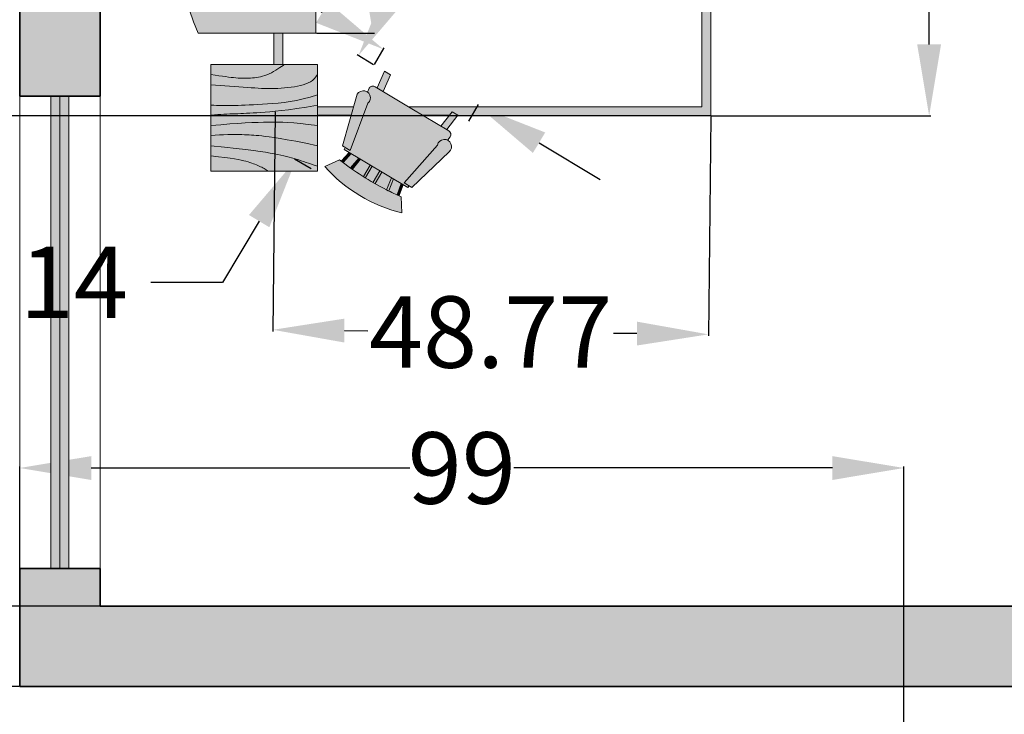
# Model space of a CAD drawing. Units: inches. Extents: x -52 to 678, y 23 to 685.
# Tile 3 of 11: x 189 to 299, y 143 to 221. Entities that reach past the tile are written whole.
import ezdxf

# ---------------------------------------------------------------- set-up
doc = ezdxf.new("R2010")
doc.units = ezdxf.units.IN
doc.header["$MEASUREMENT"] = 0
for name, color, linetype, lineweight in [('A-ANNO-DIMS', 2, 'Continuous', 18), ('A-FLOR', 7, 'Continuous', 25), ('A-FURN', 8, 'Continuous', 18), ('A-FURN-PATT', 252, 'Continuous', 13), ('A-GLAZ', 4, 'Continuous', 18), ('A-WALL', 7, 'Continuous', 35)]:
    doc.layers.add(name, color=color, linetype=linetype, lineweight=lineweight)
doc.layers.add('A-GLAZ-PATT', color=18, linetype='Continuous', lineweight=13, true_color=0x000000)
doc.layers.add('A-WALL-PATT', color=18, linetype='Continuous', lineweight=13, true_color=0x000000)
doc.styles.get("Standard").update_dxf_attribs({"font": 'arial.ttf'})
doc.dimstyles.get("Standard").update_dxf_attribs({"dimtxt": 8, "dimasz": 8, "dimexe": 0.18, "dimexo": 0.0625, "dimgap": 0.09, "dimtad": 0, "dimtih": 1, "dimtoh": 1, "dimdec": 0, "dimzin": 0, "dimdsep": 46, "dimlunit": 3, "dimtxsty": 'Standard', "dimcen": 0.09, "dimadec": 0, "dimazin": 0, "dimtfac": 1, "dimtdec": 0, "dimtofl": 0, "dimtmove": 0, "dimatfit": 3, "dimfxl": 1, "dimtolj": 1, "dimtzin": 0, "dimarcsym": 0})

# ---------------------------------------------------------------- blocks, each defined once
blk = doc.blocks.new('Table - Square Woodgrain 42 x 42 in.')
blk.add_line((0, -42), (42, -42))
for points in [[(0, -4), (1.704, -4.2172), (3.2358, -4.4188), (4.615, -4.604), (5.8615, -4.7721), (6.9951, -4.9224), (8.0357, -5.0541), (9.0031, -5.1667), (9.9171, -5.2594), (10.7951, -5.3316), (11.6445, -5.3836), (12.4702, -5.4157), (13.277, -5.4283), (14.0698, -5.4217), (14.8535, -5.3964), (15.6331, -5.3526), (16.4133, -5.2908), (17.1986, -5.2103), (17.9913, -5.1062), (18.793, -4.9727), (19.6056, -4.8038), (20.4307, -4.5937), (21.2701, -4.3365), (22.1256, -4.0262), (22.9989, -3.6571), (23.888, -3.2272), (24.7756, -2.7516), (25.6408, -2.2491), (26.4624, -1.7387), (27.2195, -1.2395), (27.891, -0.7703), (28.456, -0.3501), (28.8934, 0.002)], [(0, -42), (0, 0), (42, 0), (42, -42)], [(0, -8), (1.8203, -8.1001), (3.6741, -8.2149), (5.5411, -8.3408), (7.4011, -8.4741), (9.2339, -8.6112), (11.0193, -8.7484), (12.7371, -8.8821), (14.3671, -9.0086), (15.8954, -9.1246), (17.3337, -9.2278), (18.6997, -9.3159), (20.0116, -9.387), (21.2871, -9.4389), (22.5442, -9.4696), (23.8008, -9.477), (25.0749, -9.459), (26.3791, -9.4137), (27.7049, -9.3403), (29.0383, -9.2382), (30.3655, -9.1068), (31.6728, -8.9455), (32.9461, -8.7535), (34.1717, -8.5304), (35.3358, -8.2756), (36.4268, -7.9863), (37.443, -7.6521), (38.3849, -7.2603), (39.253, -6.7986), (40.048, -6.2542), (40.7705, -5.6147), (41.421, -4.8674), (42, -4)], [(42, -12), (39.1784, -12.8621), (36.4519, -13.5654), (33.8246, -14.1294), (31.3004, -14.5731), (28.8832, -14.9161), (26.577, -15.1775), (24.3858, -15.3768), (22.3136, -15.5332), (20.3622, -15.6632), (18.5254, -15.7718), (16.7947, -15.8612), (15.1618, -15.9338), (13.6183, -15.9916), (12.1558, -16.0369), (10.7659, -16.0718), (9.4403, -16.0987), (8.1703, -16.1191), (6.9461, -16.1325), (5.7577, -16.1377), (4.595, -16.1335), (3.4479, -16.1188), (2.3064, -16.0924), (1.1604, -16.0532), (0, -16)], [(42, -16), (37.6529, -16.7365), (33.8802, -17.329), (30.6179, -17.7961), (27.8015, -18.1561), (25.3668, -18.4275), (23.2497, -18.6288), (21.3859, -18.7785), (19.7111, -18.8949), (18.1693, -18.9939), (16.7375, -19.0795), (15.401, -19.1534), (14.1449, -19.217), (12.9544, -19.2717), (11.8148, -19.3191), (10.7113, -19.3606), (9.6291, -19.3976), (8.5534, -19.4323), (7.47, -19.4689), (6.3643, -19.5122), (5.222, -19.5672), (4.0288, -19.6386), (2.7703, -19.7313), (1.4321, -19.8501), (0, -20)], [(0, -24), (3.9243, -23.6805), (7.4766, -23.4138), (10.6891, -23.1954), (13.5943, -23.0205), (16.2247, -22.8847), (18.6125, -22.7832), (20.7903, -22.7116), (22.7903, -22.6651), (24.6563, -22.642), (26.4764, -22.6507), (28.35, -22.7024), (30.3766, -22.8084), (32.6555, -22.98), (35.2861, -23.2283), (38.3678, -23.5645), (42, -24)], [(42, -32), (37.392, -31.017), (33.4585, -30.2231), (30.1291, -29.5949), (27.3334, -29.109), (25.0009, -28.742), (23.0612, -28.4707), (21.4439, -28.2716), (20.0786, -28.1215), (18.8998, -28.0002), (17.8609, -27.9014), (16.9206, -27.8219), (16.0371, -27.7588), (15.1691, -27.709), (14.2748, -27.6693), (13.3128, -27.6368), (12.2415, -27.6083), (11.0295, -27.5824), (9.6867, -27.5643), (8.233, -27.5608), (6.6884, -27.5787), (5.0728, -27.6248), (3.4062, -27.7058), (1.7086, -27.8286), (0, -28)], [(0, -32), (5.4026, -32.5358), (9.9494, -33.019), (13.7424, -33.4553), (16.8834, -33.8505), (19.4743, -34.2106), (21.6171, -34.5413), (23.4136, -34.8486), (24.9657, -35.1382), (26.3614, -35.4156), (27.6332, -35.6841), (28.7995, -35.9467), (29.8788, -36.2064), (30.8897, -36.4661), (31.8507, -36.7288), (32.7802, -36.9973), (33.6968, -37.2747), (34.6175, -37.5635), (35.5531, -37.8651), (36.5128, -38.1805), (37.506, -38.5108), (38.5421, -38.8568), (39.6302, -39.2197), (40.7797, -39.6004), (42, -40)], [(0, -36), (3.0098, -36.2857), (5.5354, -36.5643), (7.6368, -36.8359), (9.374, -37.1009), (10.807, -37.3597), (11.9957, -37.6126), (13.0002, -37.8599), (13.8804, -38.102), (14.6874, -38.3393), (15.4365, -38.5729), (16.1338, -38.8041), (16.7858, -39.0341), (17.3987, -39.264), (17.9787, -39.4952), (18.5322, -39.7288), (19.0655, -39.9662), (19.5832, -40.2081), (20.0842, -40.4544), (20.5657, -40.7046), (21.0249, -40.9581), (21.459, -41.2144), (21.8653, -41.4731), (22.2409, -41.7335), (22.5831, -41.9951)]]:
    blk.add_lwpolyline(points)
blk = doc.blocks.new('Chair - Rocking')
for p, q in [((-8, -4.5), (-10, -1.5)), ((8, -4.5), (10, -1.5)), ((-4.5, -7), (-4.96674, -4.19951)), ((-4, -7), (-4.40532, -4.16272)), ((-1.5, -4.05012), (-1.5, -7)), ((-1, -7), (-1, -4.05012)), ((1, -7), (1, -4.04655)), ((1.5, -4.05012), (1.5, -7)), ((4, -7), (4.40187, -4.18694)), ((4.5, -7), (4.96761, -4.19437)), ((-7.5, -4.5), (-7, -7)), ((-6.5, -7), (-7.02225, -4.43)), ((6.5, -7), (7, -4.4057)), ((7.5, -4.5), (7, -7)), ((-9, -7.5), (-12, -18.49999)), ((-7, -7.5), (-9, -7.5)), ((-9, -18.49999), (-7, -7.5)), ((-8.23428, -6.99939), (-8.3093, -7.47958)), ((-8.23041, -7), (8.23915, -7)), ((7, -7.5), (9, -7.5)), ((9, -18.49999), (7, -7.5)), ((8.31071, -7.48854), (8.23449, -7.00073)), ((9, -7.5), (12, -18.49999)), ((-10.36644, -20.64523), (-10.5, -21.49999)), ((10.5, -21.49999), (10.3575, -20.58798)), ((-9, -22.49999), (-9.5, -26.49999)), ((0, -22.49999), (-9.5, -22.49999)), ((-8, -26.49999), (-7.5, -22.49999)), ((0, -22.49999), (9.5, -22.49999)), ((8, -26.49999), (7.5, -22.49999)), ((9, -22.49999), (9.5, -26.49999)), ((-9.5, -26.49999), (-8, -26.49999)), ((9.5, -26.49999), (8, -26.49999))]:
    blk.add_line(p, q)
for centre, radius, start, end in [((0, -34.08333), 34.08333, 72.93847, 107.0615), ((0, -68.25004), 64.25, 93.92211, 97.15267), ((0, -68.25004), 64.25, 82.84733, 93.92211), ((-10.5, -18.99999), 1.58114, 161.5651, 18.43495), ((10.5, -18.99999), 1.58114, 161.5651, 18.43495), ((-9.5, -21.49999), 1, 180, 270), ((9.5, -21.49999), 1, 270, 0)]:
    blk.add_arc(centre, radius, start, end)
blk = doc.blocks.new('Sofa - Roundback 7 ft.')
for p, q in [((-12.00002, -32.4421), (-12.00003, -6.5971)), ((11.99997, -32.4421), (11.99998, -6.5971)), ((-36.000027, -34), (-36.000027, -11.4696)), ((35.99998, -34), (35.99998, -11.4696)), ((-35.999844, -13.3819), (35.9998, -13.3819)), ((-36.000027, -32.4421), (35.99998, -32.4421))]:
    blk.add_line(p, q)
for points in [[(-36.000027, -34), (-42.000027, -34), (-42.000027, -8)], [(41.99998, -8), (41.99998, -34), (35.99998, -34)]]:
    blk.add_lwpolyline(points)
for centre, radius, start, end in [((0, -114.25), 114.25, 68.43141, 111.5686), ((-0.00001, -127.1968), 121.1968, 72.72033, 107.2797)]:
    blk.add_arc(centre, radius, start, end)
blk = doc.blocks.new('*D21')
at = {"layer": 'A-ANNO-DIMS', "color": 0, "lineweight": -2, "transparency": 16777216}
for p, q in [((230.65, 223.62), (234.77, 230.48)), ((228.24, 215.74), (226.38, 216.85)), ((221.23, 204.07), (219.38, 205.18)), ((215.42, 198.23), (211.3, 191.37)), ((211.3, 191.37), (203.3, 191.37))]:
    blk.add_line(p, q, dxfattribs=at)
at = {"layer": 'A-ANNO-DIMS', "color": 0, "transparency": 16777216}
for points in [[(229.51, 224.3), (231.8, 222.93), (226.54, 216.76)], [(214.28, 198.91), (216.56, 197.54), (219.54, 205.09)]]:
    blk.add_solid(points, dxfattribs=at)
at = {"layer": 'Defpoints', "color": 0, "transparency": 16777216}
for p in [(228.29, 215.71), (219.54, 205.09), (221.29, 204.04)]:
    blk.add_point(p, dxfattribs=at)
at = {"layer": 'A-ANNO-DIMS', "color": 0, "transparency": 16777216, "insert": (172.25, 191.37), "char_height": 8, "attachment_point": 5}
blk.add_mtext('\\A1;ROCKER 14', dxfattribs=at)
blk = doc.blocks.new('*D22')
at = {"layer": 'A-ANNO-DIMS', "color": 0, "lineweight": -2, "transparency": 16777216}
for p, q in [((215.62, 225.69), (207.62, 225.69)), ((222.48, 221.57), (215.62, 225.69)), ((228.32, 215.76), (229.43, 217.61)), ((238.88, 209.42), (239.99, 211.27)), ((246.76, 207), (253.62, 202.89))]:
    blk.add_line(p, q, dxfattribs=at)
at = {"layer": 'A-ANNO-DIMS', "color": 0, "transparency": 16777216}
for points in [[(223.17, 222.72), (221.79, 220.43), (229.34, 217.46)], [(247.45, 208.15), (246.07, 205.86), (239.9, 211.12)]]:
    blk.add_solid(points, dxfattribs=at)
at = {"layer": 'Defpoints', "color": 0, "transparency": 16777216}
for p in [(229.34, 217.46), (228.29, 215.71), (238.85, 209.37)]:
    blk.add_point(p, dxfattribs=at)
at = {"layer": 'A-ANNO-DIMS', "color": 0, "transparency": 16777216, "insert": (202.22, 225.69), "char_height": 8, "attachment_point": 5}
blk.add_mtext('\\A1;12', dxfattribs=at)
blk = doc.blocks.new('*D25')
at = {"layer": 'A-ANNO-DIMS', "color": 0, "lineweight": -2, "transparency": 16777216}
for p, q in [((221.83, 261.88), (228.34, 261.88)), ((228.16, 253.88), (228.16, 244.8)), ((228.16, 227.25), (228.16, 236.33)), ((221.83, 219.25), (228.34, 219.25))]:
    blk.add_line(p, q, dxfattribs=at)
at = {"layer": 'A-ANNO-DIMS', "color": 0, "transparency": 16777216}
for points in [[(226.83, 253.88), (229.49, 253.88), (228.16, 261.88)], [(226.83, 227.25), (229.49, 227.25), (228.16, 219.25)]]:
    blk.add_solid(points, dxfattribs=at)
at = {"layer": 'Defpoints', "color": 0, "transparency": 16777216}
for p in [(221.77, 261.88), (228.16, 261.88), (221.77, 219.25)]:
    blk.add_point(p, dxfattribs=at)
at = {"layer": 'A-ANNO-DIMS', "color": 0, "transparency": 16777216, "insert": (228.16, 240.57), "char_height": 8, "attachment_point": 5}
blk.add_mtext('\\A1;SOFA 43', dxfattribs=at)
blk = doc.blocks.new('*D39')
at = {"layer": 'A-ANNO-DIMS', "color": 0, "lineweight": -2, "transparency": 16777216}
for p, q in [((91.61, 327.06), (91.61, 28.49)), ((575.61, 53.06), (575.61, 28.49)), ((99.61, 28.67), (324.53, 28.67)), ((567.61, 28.67), (342.68, 28.67))]:
    blk.add_line(p, q, dxfattribs=at)
at = {"layer": 'A-ANNO-DIMS', "color": 0, "transparency": 16777216}
for points in [[(99.61, 30), (99.61, 27.33), (91.61, 28.67)], [(567.61, 30), (567.61, 27.33), (575.61, 28.67)]]:
    blk.add_solid(points, dxfattribs=at)
at = {"layer": 'Defpoints', "color": 0, "transparency": 16777216}
for p in [(91.61, 327.13), (575.61, 53.13), (575.61, 28.67)]:
    blk.add_point(p, dxfattribs=at)
at = {"layer": 'A-ANNO-DIMS', "color": 0, "transparency": 16777216, "insert": (333.61, 28.67), "char_height": 8, "attachment_point": 5}
blk.add_mtext('\\A1;484', dxfattribs=at)
blk = doc.blocks.new('*D47')
at = {"layer": 'A-ANNO-DIMS', "color": 0, "lineweight": -2, "transparency": 16777216}
for p, q in [((188.54, 146.13), (66.97, 146.13)), ((67.15, 138.13), (67.15, 103.8)), ((67.15, 61.13), (67.15, 95.45)), ((425.54, 53.13), (66.97, 53.13))]:
    blk.add_line(p, q, dxfattribs=at)
at = {"layer": 'A-ANNO-DIMS', "color": 0, "transparency": 16777216}
for points in [[(65.81, 138.13), (68.48, 138.13), (67.15, 146.13)], [(65.81, 61.13), (68.48, 61.13), (67.15, 53.13)]]:
    blk.add_solid(points, dxfattribs=at)
at = {"layer": 'Defpoints', "color": 0, "transparency": 16777216}
for p in [(67.15, 146.13), (188.61, 146.13), (425.61, 53.13)]:
    blk.add_point(p, dxfattribs=at)
at = {"layer": 'A-ANNO-DIMS', "color": 0, "transparency": 16777216, "insert": (67.15, 99.63), "char_height": 8, "attachment_point": 5}
blk.add_mtext('\\A1;93', dxfattribs=at)
blk = doc.blocks.new('*D49')
at = {"layer": 'A-ANNO-DIMS', "color": 0, "lineweight": -2, "transparency": 16777216}
for p, q in [((188.61, 146.19), (188.61, 170.77)), ((196.61, 170.59), (232.28, 170.59)), ((279.61, 170.59), (243.93, 170.59)), ((287.61, 146.19), (287.61, 170.77))]:
    blk.add_line(p, q, dxfattribs=at)
at = {"layer": 'A-ANNO-DIMS', "color": 0, "transparency": 16777216}
for points in [[(196.61, 171.92), (196.61, 169.25), (188.61, 170.59)], [(279.61, 171.92), (279.61, 169.25), (287.61, 170.59)]]:
    blk.add_solid(points, dxfattribs=at)
at = {"layer": 'Defpoints', "color": 0, "transparency": 16777216}
for p in [(287.61, 170.59), (188.61, 146.13), (287.61, 146.13)]:
    blk.add_point(p, dxfattribs=at)
at = {"layer": 'A-ANNO-DIMS', "color": 0, "transparency": 16777216, "insert": (238.11, 170.59), "char_height": 8, "attachment_point": 5}
blk.add_mtext('\\A1;99', dxfattribs=at)
blk = doc.blocks.new('*D101')
at = {"layer": 'A-ANNO-DIMS', "color": 0, "lineweight": -2, "transparency": 16777216}
for p, q in [((217.21, 210.45), (216.96, 185.88)), ((265.98, 209.95), (265.72, 185.37)), ((224.96, 185.98), (227.59, 185.95)), ((257.72, 185.64), (255.09, 185.66))]:
    blk.add_line(p, q, dxfattribs=at)
at = {"layer": 'A-ANNO-DIMS', "color": 0, "transparency": 16777216}
for points in [[(224.97, 187.31), (224.94, 184.64), (216.96, 186.06)], [(257.74, 186.97), (257.71, 184.3), (265.72, 185.55)]]:
    blk.add_solid(points, dxfattribs=at)
at = {"layer": 'Defpoints', "color": 0, "transparency": 16777216}
for p in [(217.21, 210.52), (265.98, 210.01), (216.96, 186.06)]:
    blk.add_point(p, dxfattribs=at)
at = {"layer": 'A-ANNO-DIMS', "color": 0, "transparency": 16777216, "insert": (241.34, 185.81), "char_height": 8, "attachment_point": 5}
blk.add_mtext('\\A1;48.77', dxfattribs=at)
blk = doc.blocks.new('*D102')
at = {"layer": 'A-ANNO-DIMS', "color": 0, "lineweight": -2, "transparency": 16777216}
for p, q in [((266.04, 271.64), (290.62, 271.64)), ((290.44, 263.64), (290.44, 245)), ((290.44, 218.01), (290.44, 236.65)), ((266.04, 210.01), (290.62, 210.01))]:
    blk.add_line(p, q, dxfattribs=at)
at = {"layer": 'A-ANNO-DIMS', "color": 0, "transparency": 16777216}
for points in [[(289.1, 263.64), (291.77, 263.64), (290.44, 271.64)], [(289.1, 218.01), (291.77, 218.01), (290.44, 210.01)]]:
    blk.add_solid(points, dxfattribs=at)
at = {"layer": 'Defpoints', "color": 0, "transparency": 16777216}
for p in [(265.98, 271.64), (265.98, 210.01), (290.44, 210.01)]:
    blk.add_point(p, dxfattribs=at)
at = {"layer": 'A-ANNO-DIMS', "color": 0, "transparency": 16777216, "insert": (290.44, 240.82), "char_height": 8, "attachment_point": 5}
blk.add_mtext('\\A1;61.63', dxfattribs=at)
blk = doc.blocks.new('*D104')
at = {"layer": 'A-ANNO-DIMS', "color": 0, "lineweight": -2, "transparency": 16777216}
for p, q in [((265.91, 210.01), (66.97, 210.01)), ((67.15, 202.01), (67.15, 186.74)), ((67.15, 163.13), (67.15, 178.39)), ((301.21, 155.13), (66.97, 155.13))]:
    blk.add_line(p, q, dxfattribs=at)
at = {"layer": 'A-ANNO-DIMS', "color": 0, "transparency": 16777216}
for points in [[(65.81, 202.01), (68.48, 202.01), (67.15, 210.01)], [(65.81, 163.13), (68.48, 163.13), (67.15, 155.13)]]:
    blk.add_solid(points, dxfattribs=at)
at = {"layer": 'Defpoints', "color": 0, "transparency": 16777216}
for p in [(265.98, 210.01), (67.15, 155.13), (301.27, 155.13)]:
    blk.add_point(p, dxfattribs=at)
at = {"layer": 'A-ANNO-DIMS', "color": 0, "transparency": 16777216, "insert": (67.15, 182.57), "char_height": 8, "attachment_point": 5}
blk.add_mtext('\\A1;54.89', dxfattribs=at)

msp = doc.modelspace()

# ---------------------------------------------------------------- hatches: boundary and pattern name
at = {"layer": 'A-FURN-PATT'}
h = msp.add_hatch(color=256, dxfattribs=at)
h.dxf.hatch_style = 1
h.paths.add_polyline_path([(264.9763, 211.0118), (232.1935, 211.0118), (232.532, 210.8087), (233.7567, 210.0739), (236.7223, 210.0739), (237.0272, 210.4629), (237.6755, 210.0739), (265.9763, 210.0118), (265.9763, 211.0118), (265.9763, 271.638), (264.9763, 271.638), (252.0267, 271.638), (252.0267, 270.638), (264.9763, 270.638)])
h = msp.add_hatch(color=256, dxfattribs=at)
h.dxf.hatch_style = 1
h.paths.add_polyline_path([(221.7669, 219.2523), (221.7669, 222.2971), (210.3335, 222.2971, -0.15194781), (210.3335, 258.8353), (221.7669, 258.8353), (221.7669, 261.8802), (208.5725, 261.8802, 0.19047621), (208.5725, 219.2523)])
h = msp.add_hatch(color=256, dxfattribs=at)
h.dxf.hatch_style = 1
h.paths.add_polyline_path([(218.0681, 219.2523), (217.0681, 219.2523), (217.0681, 215.7592), (218.0681, 215.7592)])
h = msp.add_hatch(color=256, dxfattribs=at)
h.dxf.hatch_style = 1
h.paths.add_polyline_path([(214.8875, 214.2771), (215.113, 214.3067), (215.3411, 214.3447), (215.5722, 214.3927), (215.8069, 214.4525), (216.0457, 214.5257), (216.2891, 214.6139), (216.5375, 214.7189), (216.7904, 214.8412), (217.0429, 214.9765), (217.289, 215.1195), (217.5227, 215.2646), (217.7381, 215.4066), (217.9291, 215.5401), (218.0898, 215.6596), (218.2135, 215.7592), (209.9953, 215.7592), (209.9953, 214.6214), (210.48, 214.5596), (210.9157, 214.5023), (211.308, 214.4496), (211.6626, 214.4018), (211.9851, 214.359), (212.2811, 214.3215), (212.5563, 214.2895), (212.8163, 214.2631), (213.066, 214.2426), (213.3076, 214.2278), (213.5425, 214.2187), (213.772, 214.2151), (213.9975, 214.217), (214.2205, 214.2242), (214.4422, 214.2366), (214.6642, 214.2542)])
h = msp.add_hatch(color=256, dxfattribs=at)
h.dxf.hatch_style = 1
h.paths.add_polyline_path([(217.499, 213.0814), (217.8762, 213.1023), (218.2555, 213.1313), (218.633, 213.1687), (219.0049, 213.2146), (219.3671, 213.2692), (219.7157, 213.3327), (220.0468, 213.4052), (220.3572, 213.4875), (220.6462, 213.5825), (220.9142, 213.694), (221.1611, 213.8253), (221.3873, 213.9802), (221.5928, 214.1621), (221.7778, 214.3747), (221.9425, 214.6214), (221.9425, 215.7592), (218.2135, 215.7592), (218.0898, 215.6596), (217.9291, 215.5401), (217.7381, 215.4066), (217.5227, 215.2646), (217.289, 215.1195), (217.0429, 214.9765), (216.7904, 214.8412), (216.5375, 214.7189), (216.2891, 214.6139), (216.0457, 214.5257), (215.8069, 214.4525), (215.5722, 214.3927), (215.3411, 214.3447), (215.113, 214.3067), (214.8875, 214.2771), (214.6642, 214.2542), (214.4422, 214.2366), (214.2205, 214.2242), (213.9975, 214.217), (213.772, 214.2151), (213.5425, 214.2187), (213.3076, 214.2278), (213.066, 214.2426), (212.8163, 214.2631), (212.5563, 214.2895), (212.2811, 214.3215), (211.9851, 214.359), (211.6626, 214.4018), (211.308, 214.4496), (210.9157, 214.5023), (210.48, 214.5596), (209.9953, 214.6214), (209.9953, 213.4836), (210.5131, 213.4551), (211.0404, 213.4224), (211.5715, 213.3866), (212.1006, 213.3487), (212.6219, 213.3097), (213.1298, 213.2707), (213.6184, 213.2326), (214.0821, 213.1967), (214.5168, 213.1637), (214.926, 213.1343), (215.3145, 213.1092), (215.6877, 213.089), (216.0506, 213.0742), (216.4081, 213.0655), (216.7656, 213.0634), (217.128, 213.0685)])
h = msp.add_hatch(color=256, dxfattribs=at)
h.dxf.hatch_style = 1
h.paths.add_polyline_path([(230.1116, 214.6122), (229.4633, 215.0012), (228.642, 213.1427), (229.2904, 212.7537)])
h = msp.add_hatch(color=256, dxfattribs=at)
h.dxf.hatch_style = 1
h.paths.add_polyline_path([(214.926, 213.1343), (214.5168, 213.1637), (214.0821, 213.1967), (213.6184, 213.2326), (213.1298, 213.2707), (212.6219, 213.3097), (212.1006, 213.3487), (211.5715, 213.3866), (211.0404, 213.4224), (210.5131, 213.4551), (209.9953, 213.4836), (209.9953, 211.2079), (210.3253, 211.1928), (210.6513, 211.1816), (210.976, 211.1741), (211.3023, 211.1699), (211.6331, 211.1687), (211.9711, 211.1702), (212.3194, 211.174), (212.6806, 211.1798), (213.0577, 211.1875), (213.4531, 211.1974), (213.8691, 211.2103), (214.3082, 211.2267), (214.7727, 211.2474), (215.265, 211.2728), (215.7875, 211.3037), (216.3426, 211.3407), (216.932, 211.3852), (217.5553, 211.4419), (218.2113, 211.5162), (218.8989, 211.6138), (219.617, 211.74), (220.3643, 211.9004), (221.1399, 212.1005), (221.9425, 212.3457), (221.9425, 214.6214), (221.7778, 214.3747), (221.5928, 214.1621), (221.3873, 213.9802), (221.1611, 213.8253), (220.9142, 213.694), (220.6462, 213.5825), (220.3572, 213.4875), (220.0468, 213.4052), (219.7157, 213.3327), (219.3671, 213.2692), (219.0049, 213.2146), (218.633, 213.1687), (218.2555, 213.1313), (217.8762, 213.1023), (217.499, 213.0814), (217.128, 213.0685), (216.7656, 213.0634), (216.4081, 213.0655), (216.0506, 213.0742), (215.6877, 213.089), (215.3145, 213.1092)])
h = msp.add_hatch(color=256, dxfattribs=at)
h.dxf.hatch_style = 1
h.paths.add_polyline_path([(224.752, 206.6593), (225.6165, 206.1406), (227.6047, 211.4138, 1.38742744), (226.308, 212.1918)])
h = msp.add_hatch(color=256, dxfattribs=at)
h.dxf.hatch_style = 1
h.paths.add_polyline_path([(228.4259, 213.2723, 0.41421356), (227.7344, 213.0994), (227.5568, 212.6619, -0.48335183), (227.6047, 211.4138), (225.6165, 206.1406), (225.0492, 206.481), (224.9533, 206.2446), (232.0715, 201.9737), (232.2349, 202.1696), (231.6676, 202.51), (235.3847, 206.7457, -0.4833507), (236.5085, 207.2909), (236.8111, 207.6534, 0.41421356), (236.6382, 208.345), (232.532, 210.8087)])
h = msp.add_hatch(color=256, dxfattribs=at)
h.dxf.hatch_style = 1
h.paths.add_polyline_path([(215.6022, 210.3844), (216.0787, 210.4175), (216.6088, 210.4601), (217.2111, 210.5174), (217.9036, 210.5946), (218.7048, 210.697), (219.6328, 210.8298), (220.706, 210.9984), (221.9425, 211.2079), (221.9425, 212.3457), (221.1399, 212.1005), (220.3643, 211.9004), (219.617, 211.74), (218.8989, 211.6138), (218.2113, 211.5162), (217.5553, 211.4419), (216.932, 211.3852), (216.3426, 211.3407), (215.7875, 211.3037), (215.265, 211.2728), (214.7727, 211.2474), (214.3082, 211.2267), (213.8691, 211.2103), (213.4531, 211.1974), (213.0577, 211.1875), (212.6806, 211.1798), (212.3194, 211.174), (211.9711, 211.1702), (211.6331, 211.1687), (211.3023, 211.1699), (210.976, 211.1741), (210.6513, 211.1816), (210.3253, 211.1928), (209.9953, 211.2079), (209.9953, 210.0701), (210.4026, 210.1127), (210.7833, 210.1465), (211.1413, 210.1729), (211.4807, 210.1932), (211.8056, 210.2088), (212.1202, 210.2211), (212.4283, 210.2315), (212.7343, 210.2414), (213.0422, 210.2519), (213.3561, 210.2637), (213.6802, 210.2772), (214.0189, 210.2928), (214.3762, 210.3109), (214.7564, 210.3319), (215.1637, 210.3562)])
h = msp.add_hatch(color=256, dxfattribs=at)
h.dxf.hatch_style = 1
h.paths.add_polyline_path([(215.9092, 209.2987), (216.4782, 209.3119), (217.009, 209.3185), (217.5267, 209.316), (218.0597, 209.3013), (218.6361, 209.2712), (219.2844, 209.2224), (220.0327, 209.1517), (220.9093, 209.0561), (221.9425, 208.9322), (221.9425, 211.2079), (220.706, 210.9984), (219.6328, 210.8298), (218.7048, 210.697), (217.9036, 210.5946), (217.2111, 210.5174), (216.6088, 210.4601), (216.0787, 210.4175), (215.6022, 210.3844), (215.1637, 210.3562), (214.7564, 210.3319), (214.3762, 210.3109), (214.0189, 210.2928), (213.6802, 210.2772), (213.3561, 210.2637), (213.0422, 210.2519), (212.7343, 210.2414), (212.4283, 210.2315), (212.1202, 210.2211), (211.8056, 210.2088), (211.4807, 210.1932), (211.1413, 210.1729), (210.7833, 210.1465), (210.4026, 210.1127), (209.9953, 210.0701), (209.9953, 208.9322), (211.1116, 209.0231), (212.122, 209.099), (213.0359, 209.1611), (213.8623, 209.2108), (214.6105, 209.2495), (215.2897, 209.2783)])
h = msp.add_hatch(color=256, dxfattribs=at)
h.dxf.hatch_style = 1
h.paths.add_polyline_path([(225.7124, 210.0739), (225.9761, 211.0118), (221.9425, 211.0118), (221.9425, 210.0739)])
h = msp.add_hatch(color=256, dxfattribs=at)
h.dxf.hatch_style = 1
h.paths.add_polyline_path([(235.7737, 208.8636), (236.4221, 208.4746), (237.6755, 210.0739), (237.0272, 210.4629)])
h = msp.add_hatch(color=256, dxfattribs=at)
h.dxf.hatch_style = 1
h.paths.add_polyline_path([(215.9092, 209.2987), (215.2897, 209.2783), (214.6105, 209.2495), (213.8623, 209.2108), (213.0359, 209.1611), (212.122, 209.099), (211.1116, 209.0231), (209.9953, 208.9322), (209.9953, 207.7944), (210.4813, 207.8431), (210.9642, 207.8781), (211.4383, 207.9011), (211.8978, 207.9142), (212.3372, 207.9193), (212.7507, 207.9183), (213.1327, 207.9132), (213.4775, 207.9058), (213.7822, 207.8977), (214.0558, 207.8885), (214.3102, 207.8772), (214.5571, 207.863), (214.8085, 207.845), (215.0759, 207.8224), (215.3715, 207.7943), (215.7068, 207.7598), (216.0952, 207.7171), (216.5552, 207.6605), (217.107, 207.5833), (217.7705, 207.4789), (218.5657, 207.3407), (219.5128, 207.162), (220.6317, 206.9362), (221.9425, 206.6565), (221.9425, 208.9322), (220.9093, 209.0561), (220.0327, 209.1517), (219.2844, 209.2224), (218.6361, 209.2712), (218.0597, 209.3013), (217.5267, 209.316), (217.009, 209.3185), (216.4782, 209.3119)])
h = msp.add_hatch(color=256, dxfattribs=at)
h.dxf.hatch_style = 1
h.paths.add_polyline_path([(215.7068, 207.7598), (215.3715, 207.7943), (215.0759, 207.8224), (214.8085, 207.845), (214.5571, 207.863), (214.3102, 207.8772), (214.0558, 207.8885), (213.7822, 207.8977), (213.4775, 207.9058), (213.1327, 207.9132), (212.7507, 207.9183), (212.3372, 207.9193), (211.8978, 207.9142), (211.4383, 207.9011), (210.9642, 207.8781), (210.4813, 207.8431), (209.9953, 207.7944), (209.9953, 206.6565), (211.5321, 206.5041), (212.8254, 206.3667), (213.9044, 206.2426), (214.7979, 206.1302), (215.5349, 206.0277), (216.1444, 205.9337), (216.6555, 205.8462), (217.097, 205.7639), (217.494, 205.6849), (217.8558, 205.6086), (218.1875, 205.5339), (218.4945, 205.46), (218.7821, 205.3861), (219.0555, 205.3114), (219.3199, 205.235), (219.5806, 205.1561), (219.8425, 205.074), (220.1086, 204.9882), (220.3816, 204.8984), (220.6642, 204.8045), (220.9589, 204.7061), (221.2684, 204.6028), (221.5954, 204.4945), (221.9425, 204.3809), (221.9425, 206.6565), (220.6317, 206.9362), (219.5128, 207.162), (218.5657, 207.3407), (217.7705, 207.4789), (217.107, 207.5833), (216.5552, 207.6605), (216.0952, 207.7171)])
h = msp.add_hatch(color=256, dxfattribs=at)
h.dxf.hatch_style = 1
h.paths.add_polyline_path([(236.6814, 205.9677, 1.38742744), (235.3847, 206.7457), (231.6676, 202.51), (232.532, 201.9913)])
h = msp.add_hatch(color=256, dxfattribs=at)
h.dxf.hatch_style = 1
h.paths.add_polyline_path([(216.1444, 205.9337), (215.5349, 206.0277), (214.7979, 206.1302), (213.9044, 206.2426), (212.8254, 206.3667), (211.5321, 206.5041), (209.9953, 206.6565), (209.9953, 205.5187), (210.8514, 205.4374), (211.5698, 205.3582), (212.1676, 205.2809), (212.6618, 205.2055), (213.0694, 205.1319), (213.4075, 205.06), (213.6933, 204.9896), (213.9437, 204.9208), (214.1732, 204.8533), (214.3863, 204.7868), (214.5847, 204.7211), (214.7701, 204.6556), (214.9445, 204.5902), (215.1095, 204.5245), (215.2669, 204.458), (215.4186, 204.3905), (215.5659, 204.3217), (215.7084, 204.2516), (215.8453, 204.1804), (215.976, 204.1083), (216.0995, 204.0354), (216.215, 203.9618), (216.3219, 203.8878), (216.421, 203.812), (221.9425, 203.812), (221.9425, 204.3809), (221.5954, 204.4945), (221.2684, 204.6028), (220.9589, 204.7061), (220.6642, 204.8045), (220.3816, 204.8984), (220.1086, 204.9882), (219.8425, 205.074), (219.5806, 205.1561), (219.3199, 205.235), (219.0555, 205.3114), (218.7821, 205.3861), (218.4945, 205.46), (218.1875, 205.5339), (217.8558, 205.6086), (217.494, 205.6849), (217.097, 205.7639), (216.6555, 205.8462)])
h = msp.add_hatch(color=256, dxfattribs=at)
h.dxf.hatch_style = 1
h.paths.add_polyline_path([(211.5698, 205.3582), (210.8514, 205.4374), (209.9953, 205.5187), (209.9953, 203.812), (216.421, 203.812), (216.3219, 203.8878), (216.215, 203.9618), (216.0995, 204.0354), (215.976, 204.1083), (215.8453, 204.1804), (215.7084, 204.2516), (215.5659, 204.3217), (215.4186, 204.3905), (215.2669, 204.458), (215.1095, 204.5245), (214.9445, 204.5902), (214.7701, 204.6556), (214.5847, 204.7211), (214.3863, 204.7868), (214.1732, 204.8533), (213.9437, 204.9208), (213.6933, 204.9896), (213.4075, 205.06), (213.0694, 205.1319), (212.6618, 205.2055), (212.1676, 205.2809)])
h = msp.add_hatch(color=256, dxfattribs=at)
h.dxf.hatch_style = 1
h.paths.add_polyline_path([(229.6729, 201.7379, -0.04836039), (224.4062, 205.1033), (222.7638, 204.3253, 0.15000001), (231.4083, 199.1386), (231.3218, 200.954, -0.01409681)])
h = msp.add_hatch(color=256, dxfattribs=at)
h.dxf.hatch_style = 1
h.paths.add_polyline_path([(225.7029, 205.7949), (225.4868, 205.9245), (224.6018, 204.9511, 0.00198738), (224.8062, 204.7945)])
h = msp.add_hatch(color=256, dxfattribs=at)
h.dxf.hatch_style = 1
h.paths.add_polyline_path([(224.8062, 204.7945, 0.00795902), (225.637, 204.184), (226.5673, 205.2762), (225.7029, 205.7949)])
h = msp.add_hatch(color=256, dxfattribs=at)
h.dxf.hatch_style = 1
h.paths.add_polyline_path([(226.5673, 205.2762), (225.637, 204.184, 0.03647942), (229.6729, 201.7379, 0.00223634), (229.9315, 201.6073), (230.4574, 202.9422)])
h = msp.add_hatch(color=256, dxfattribs=at)
h.dxf.hatch_style = 1
h.paths.add_polyline_path([(225.637, 204.184, 0.00218867), (225.8688, 204.0208), (226.7835, 205.1465), (226.5673, 205.2762)])
h = msp.add_hatch(color=256, dxfattribs=at)
h.dxf.hatch_style = 1
h.paths.add_polyline_path([(228.0801, 204.3685), (227.864, 204.4982), (227.0906, 203.2091, 0.0019459), (227.3042, 203.0752)])
h = msp.add_hatch(color=256, dxfattribs=at)
h.dxf.hatch_style = 1
h.paths.add_polyline_path([(228.1686, 202.5566, 0.0019459), (228.3872, 202.4311), (229.1607, 203.7202), (228.9446, 203.8499)])
h = msp.add_hatch(color=256, dxfattribs=at)
h.dxf.hatch_style = 1
h.paths.add_polyline_path([(230.4574, 202.9422), (230.2413, 203.0718), (229.6784, 201.7351, 0.00218866), (229.9315, 201.6073)])
h = msp.add_hatch(color=256, dxfattribs=at)
h.dxf.hatch_style = 1
h.paths.add_polyline_path([(230.4574, 202.9422), (230.2413, 203.0718), (229.6784, 201.7351, 0.00218866), (229.9315, 201.6073)])
h = msp.add_hatch(color=256, dxfattribs=at)
h.dxf.hatch_style = 1
h.paths.add_polyline_path([(229.9315, 201.6073, 0.00806409), (230.8735, 201.1559), (231.3218, 202.4235), (230.4574, 202.9422)])
h = msp.add_hatch(color=256, dxfattribs=at)
h.dxf.hatch_style = 1
h.paths.add_polyline_path([(231.5379, 202.2938), (231.3218, 202.4235), (230.8735, 201.1559, 0.00188237), (231.0954, 201.0549)])
at = {"layer": 'A-GLAZ-PATT'}
h = msp.add_hatch(color=256, dxfattribs=at)
h.dxf.hatch_style = 1
h.paths.add_polyline_path([(193.1053, 212.2126), (192.1053, 212.2126), (192.1053, 159.3213), (193.1053, 159.3213)])
h = msp.add_hatch(color=256, dxfattribs=at)
h.dxf.hatch_style = 1
h.paths.add_polyline_path([(193.1053, 159.3213), (194.1053, 159.3213), (194.1053, 212.2126), (193.1053, 212.2126)])
at = {"layer": 'A-WALL-PATT'}
h = msp.add_hatch(color=256, dxfattribs=at)
h.dxf.hatch_style = 1
h.paths.add_polyline_path([(188.6053, 212.2126), (197.6053, 212.2126), (197.6053, 266.1726), (188.6053, 266.1726)])
h = msp.add_hatch(color=256, dxfattribs=at)
h.dxf.hatch_style = 1
h.paths.add_polyline_path([(301.2728, 146.1267), (301.2728, 155.1267), (197.6053, 155.1267), (197.6053, 159.3213), (188.6053, 159.3213), (188.6053, 146.1267)])

# ---------------------------------------------------------------- linework, layer by layer
at = {"layer": 'A-FLOR'}
msp.add_line((287.6053, 54.6267), (287.6053, 146.1267), dxfattribs=at)
at = {"layer": 'A-FURN'}
for p, q in [((265.9763, 271.638), (265.9763, 210.0118)), ((264.9763, 270.638), (264.9763, 211.0118)), ((217.0681, 219.2523), (217.0681, 215.7592)), ((218.0681, 219.2523), (218.0681, 215.7592)), ((225.9761, 211.0118), (221.9425, 211.0118)), ((264.9763, 211.0118), (232.1935, 211.0118)), ((265.9763, 210.0118), (265.9763, 211.0118)), ((225.7124, 210.0739), (221.9425, 210.0739)), ((236.7223, 210.0739), (233.7567, 210.0739)), ((265.9763, 210.0118), (237.6755, 210.0739))]:
    msp.add_line(p, q, dxfattribs=at)
at = {"layer": 'A-GLAZ'}
for p, q in [((188.6053, 159.3213), (188.6053, 212.2126)), ((192.1053, 159.3213), (192.1053, 212.2126)), ((193.1053, 159.3213), (193.1053, 212.2126)), ((194.1053, 159.3213), (194.1053, 212.2126)), ((197.6053, 159.3213), (197.6053, 212.2126))]:
    msp.add_line(p, q, dxfattribs=at)
at = {"layer": 'A-WALL'}
for p, q in [((188.6053, 212.2126), (188.6053, 266.1726)), ((197.6053, 212.2126), (197.6053, 266.1726)), ((197.6053, 212.2126), (188.6053, 212.2126)), ((188.6053, 146.1267), (188.6053, 159.3213)), ((197.6053, 159.3213), (188.6053, 159.3213)), ((197.6053, 155.1267), (197.6053, 159.3213)), ((197.6053, 155.1267), (301.2728, 155.1267)), ((188.6053, 146.1267), (301.2728, 146.1267))]:
    msp.add_line(p, q, dxfattribs=at)

# ---------------------------------------------------------------- block references
at = {"layer": 'A-FURN'}
for name, p, xscale, yscale, zscale, rotation in [('Sofa - Roundback 7 ft.', (204.5127, 240.5662), 0.5074751266368834, 0.5074751266368834, 0.5074751266368834, 90), ('Chair - Rocking', (226.697, 201.0836), 0.5040555194766858, 0.5040555194766858, 0.5040555194766858, 149.0362133943827)]:
    msp.add_blockref(name, p, dxfattribs=dict(at, xscale=xscale, yscale=yscale, zscale=zscale, rotation=rotation))
at = {"layer": 'A-FURN', "xscale": 0.2844588312427021, "yscale": 0.2844588312427021, "zscale": 0.2844588312427021}
msp.add_blockref('Table - Square Woodgrain 42 x 42 in.', (209.9953, 215.7592), dxfattribs=at)

# ---------------------------------------------------------------- dimensions: what is measured, and where the dimension line sits
at = {"layer": 'A-ANNO-DIMS'}
for base, p1, p2, picture, middle in [((575.6053, 28.6667), (91.6053, 327.1267), (575.6053, 53.1267), '*D39', (333.6053, 28.6667)), ((287.6053, 170.5867), (188.6053, 146.1267), (287.6053, 146.1267), '*D49', (238.1053, 170.5867))]:
    dim = msp.add_linear_dim(base=base, p1=p1, p2=p2, dimstyle='Standard', override={"dimdec": 0, "dimlfac": 1, "dimrnd": 0, "dimzin": 0, "dimdsep": 46, "dimlunit": 2}, dxfattribs=at)
    dim.commit()
    dim.dimension.update_dxf_attribs({"geometry": picture, "text_midpoint": middle})
for base, p1, p2, angle, override, picture, middle in [((290.4363, 210.0118), (265.9763, 271.638), (265.9763, 210.0118), 270, {"dimdec": 2, "dimlfac": 1, "dimrnd": 0, "dimzin": 0, "dimdsep": 46, "dimlunit": 2}, '*D102', (290.4363, 240.8249)), ((229.339, 217.4565), (238.8501, 209.3691), (228.2887, 215.706), 149.036213, {"dimdec": 0, "dimlfac": 1, "dimrnd": 0, "dimzin": 0, "dimdsep": 46, "dimlunit": 2}, '*D22', (202.2167, 225.6884)), ((67.1453, 155.1267), (265.9763, 210.0118), (301.2728, 155.1267), 90, {"dimdec": 2, "dimlfac": 1, "dimrnd": 0, "dimzin": 0, "dimdsep": 46, "dimlunit": 2}, '*D104', (67.1453, 182.5693)), ((216.9575, 186.0587), (265.9763, 210.0118), (217.2111, 210.5174), 179.40598, {"dimdec": 2, "dimlfac": 1, "dimrnd": 0, "dimzin": 0, "dimdsep": 46, "dimlunit": 2}, '*D101', (241.3401, 185.8059)), ((67.1453, 146.1267), (425.6053, 53.1267), (188.6053, 146.1267), 90, {"dimdec": 0, "dimlfac": 1, "dimrnd": 0, "dimzin": 0, "dimdsep": 46, "dimlunit": 2}, '*D47', (67.1453, 99.6267))]:
    dim = msp.add_linear_dim(base=base, p1=p1, p2=p2, angle=angle, dimstyle='Standard', override=override, dxfattribs=at)
    dim.commit()
    dim.dimension.update_dxf_attribs({"geometry": picture, "text_midpoint": middle})
for base, p1, p2, angle, text, picture, middle in [((228.1611, 261.8802), (221.7669, 219.2523), (221.7669, 261.8802), 90, 'SOFA <>', '*D25', (228.1611, 240.5662)), ((219.5361, 205.0862), (228.2887, 215.706), (221.2866, 204.0359), 239.036213, 'ROCKER <>', '*D21', (172.2483, 191.3664))]:
    dim = msp.add_linear_dim(base=base, p1=p1, p2=p2, angle=angle, text=text, dimstyle='Standard', override={"dimdec": 0, "dimlfac": 1, "dimrnd": 0, "dimzin": 0, "dimdsep": 46, "dimlunit": 2}, dxfattribs=at)
    dim.commit()
    dim.dimension.update_dxf_attribs({"geometry": picture, "text_midpoint": middle})

doc.saveas('drawing.dxf')
